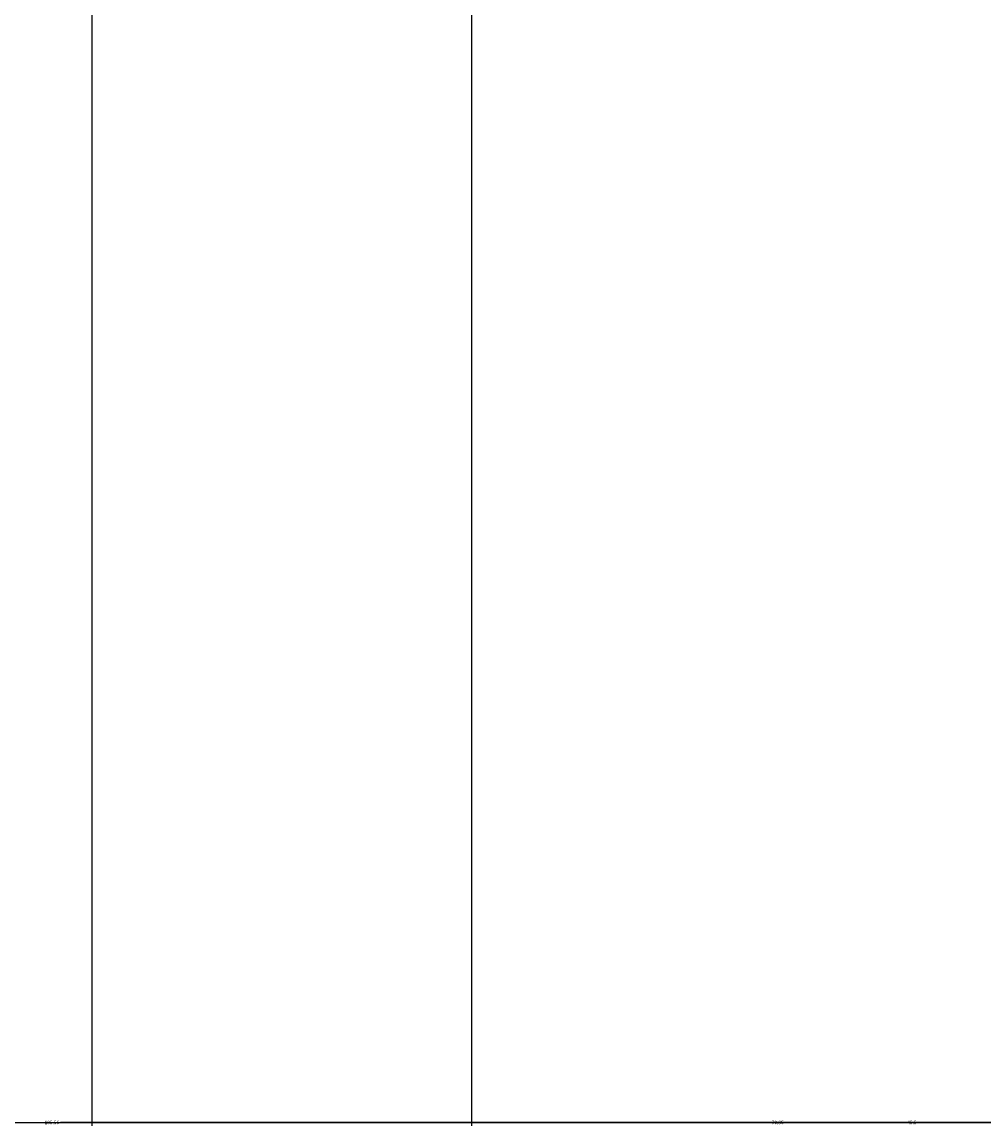
# Model space of a CAD drawing. Units: inches. Extents: x 738 to 1068, y 378 to 757.
# Tile 11 of 41: x 833 to 882, y 378 to 435. Entities that reach past the tile are written whole.
import ezdxf

# ---------------------------------------------------------------- set-up
doc = ezdxf.new("R2010")
doc.units = ezdxf.units.IN
doc.header["$MEASUREMENT"] = 0
doc.layers.add('A-ANNO-DIMS', color=2, linetype='Continuous', lineweight=18)
doc.styles.get("Standard").update_dxf_attribs({"font": 'arial.ttf'})
doc.dimstyles.get("Standard").update_dxf_attribs({"dimtxt": 0.18, "dimasz": 0.18, "dimexe": 0.18, "dimexo": 0.0625, "dimgap": 0.09, "dimtad": 0, "dimtih": 1, "dimtoh": 1, "dimdec": 4, "dimzin": 0, "dimdsep": 46, "dimtxsty": 'Standard', "dimcen": 0.09, "dimadec": 0, "dimazin": 0, "dimtfac": 1, "dimtdec": 4, "dimtofl": 0, "dimtmove": 0, "dimatfit": 3, "dimfxl": 1, "dimtolj": 1, "dimtzin": 0, "dimarcsym": 0})

# ---------------------------------------------------------------- blocks, each defined once
blk = doc.blocks.new('*D17')
at = {"layer": 'A-ANNO-DIMS', "color": 0, "lineweight": -2, "transparency": 16777216}
for p, q in [((756.324, 415.842), (756.324, 378.239)), ((1050.049, 415.919), (1050.049, 378.239)), ((756.504, 378.419), (902.791, 378.419)), ((1049.869, 378.419), (903.582, 378.419))]:
    blk.add_line(p, q, dxfattribs=at)
at = {"layer": 'A-ANNO-DIMS', "color": 0, "transparency": 16777216}
for points in [[(756.504, 378.449), (756.504, 378.389), (756.324, 378.419)], [(1049.869, 378.449), (1049.869, 378.389), (1050.049, 378.419)]]:
    blk.add_solid(points, dxfattribs=at)
at = {"layer": 'Defpoints', "color": 0, "transparency": 16777216}
for p in [(756.324, 415.904), (1050.049, 415.982), (1050.049, 378.419)]:
    blk.add_point(p, dxfattribs=at)
at = {"layer": 'A-ANNO-DIMS', "color": 0, "transparency": 16777216, "insert": (903.186, 378.419), "char_height": 0.18, "attachment_point": 5}
blk.add_mtext('\\A1;293.7', dxfattribs=at)
blk = doc.blocks.new('*D33')
at = {"layer": 'A-ANNO-DIMS', "color": 0, "lineweight": -2, "transparency": 16777216}
for p, q in [((836.324, 514.624), (836.324, 378.239)), ((907.171, 514.624), (907.171, 378.239)), ((836.504, 378.419), (871.354, 378.419)), ((906.991, 378.419), (872.141, 378.419))]:
    blk.add_line(p, q, dxfattribs=at)
at = {"layer": 'A-ANNO-DIMS', "color": 0, "transparency": 16777216}
for points in [[(836.504, 378.449), (836.504, 378.389), (836.324, 378.419)], [(906.991, 378.449), (906.991, 378.389), (907.171, 378.419)]]:
    blk.add_solid(points, dxfattribs=at)
at = {"layer": 'Defpoints', "color": 0, "transparency": 16777216}
for p in [(836.324, 514.687), (907.171, 514.687), (907.171, 378.419)]:
    blk.add_point(p, dxfattribs=at)
at = {"layer": 'A-ANNO-DIMS', "color": 0, "transparency": 16777216, "insert": (871.748, 378.419), "char_height": 0.18, "attachment_point": 5}
blk.add_mtext('\\A1;70.85', dxfattribs=at)
blk = doc.blocks.new('*D35')
at = {"layer": 'A-ANNO-DIMS', "color": 0, "lineweight": -2, "transparency": 16777216}
for p, q in [((855.932, 686.266), (855.932, 378.239)), ((901.429, 686.267), (901.429, 378.239)), ((856.112, 378.419), (878.352, 378.419)), ((901.249, 378.419), (879.009, 378.419))]:
    blk.add_line(p, q, dxfattribs=at)
at = {"layer": 'A-ANNO-DIMS', "color": 0, "transparency": 16777216}
for points in [[(856.112, 378.449), (856.112, 378.389), (855.932, 378.419)], [(901.249, 378.449), (901.249, 378.389), (901.429, 378.419)]]:
    blk.add_solid(points, dxfattribs=at)
at = {"layer": 'Defpoints', "color": 0, "transparency": 16777216}
for p in [(855.932, 686.329), (901.429, 686.329), (901.429, 378.419)]:
    blk.add_point(p, dxfattribs=at)
at = {"layer": 'A-ANNO-DIMS', "color": 0, "transparency": 16777216, "insert": (878.68, 378.419), "char_height": 0.18, "attachment_point": 5}
blk.add_mtext('\\A1;45.5', dxfattribs=at)
blk = doc.blocks.new('*D38')
at = {"layer": 'A-ANNO-DIMS', "color": 0, "lineweight": -2, "transparency": 16777216}
for p, q in [((781.485, 593.017), (781.485, 378.239)), ((887.04, 593.067), (887.04, 378.239)), ((781.665, 378.419), (833.807, 378.419)), ((886.86, 378.419), (834.718, 378.419))]:
    blk.add_line(p, q, dxfattribs=at)
at = {"layer": 'A-ANNO-DIMS', "color": 0, "transparency": 16777216}
for points in [[(781.665, 378.449), (781.665, 378.389), (781.485, 378.419)], [(886.86, 378.449), (886.86, 378.389), (887.04, 378.419)]]:
    blk.add_solid(points, dxfattribs=at)
at = {"layer": 'Defpoints', "color": 0, "transparency": 16777216}
for p in [(781.485, 593.08), (887.04, 593.13), (887.04, 378.419)]:
    blk.add_point(p, dxfattribs=at)
at = {"layer": 'A-ANNO-DIMS', "color": 0, "transparency": 16777216, "insert": (834.263, 378.419), "char_height": 0.18, "attachment_point": 5}
blk.add_mtext('\\A1;105.56', dxfattribs=at)

msp = doc.modelspace()

# ---------------------------------------------------------------- dimensions: what is measured, and where the dimension line sits
at = {"layer": 'A-ANNO-DIMS'}
for base, p1, p2, override, picture, middle in [((901.4286, 378.4191), (855.9323, 686.329), (901.4286, 686.3292), {"dimdec": 1, "dimlfac": 1, "dimrnd": 0, "dimzin": 0, "dimdsep": 46, "dimlunit": 2}, '*D35', (878.6804, 378.4191)), ((887.0404, 378.4191), (781.4846, 593.0796), (887.0404, 593.1296), {"dimdec": 2, "dimlfac": 1, "dimrnd": 0, "dimzin": 0, "dimdsep": 46, "dimlunit": 2}, '*D38', (834.2625, 378.4191)), ((907.1708, 378.4191), (836.3244, 514.6866), (907.1708, 514.6866), {"dimdec": 2, "dimlfac": 1, "dimrnd": 0, "dimzin": 0, "dimdsep": 46, "dimlunit": 2}, '*D33', (871.7476, 378.4191)), ((1050.0492, 378.4191), (756.3236, 415.904), (1050.0492, 415.982), {"dimdec": 1, "dimlfac": 1, "dimrnd": 0, "dimzin": 0, "dimdsep": 46, "dimlunit": 2}, '*D17', (903.1864, 378.4191))]:
    dim = msp.add_linear_dim(base=base, p1=p1, p2=p2, dimstyle='Standard', override=override, dxfattribs=at)
    dim.commit()
    dim.dimension.update_dxf_attribs({"geometry": picture, "text_midpoint": middle})

doc.saveas('drawing.dxf')
